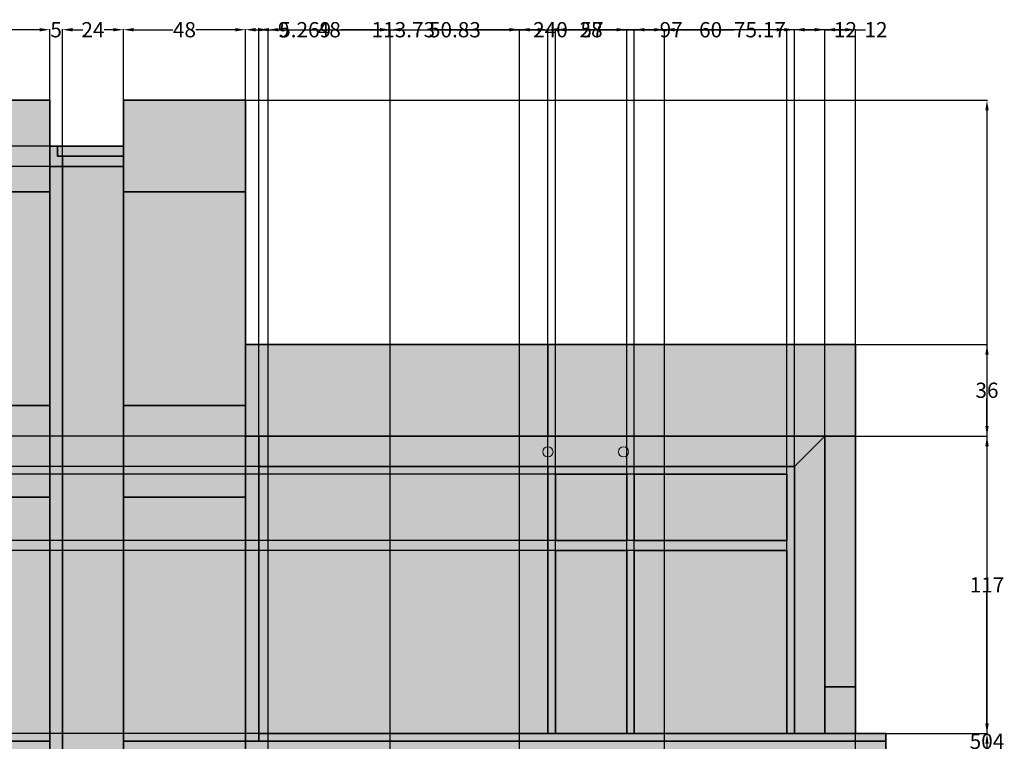
# Model space of a CAD drawing. Units: inches. Extents: x 221 to 874, y 171 to 738.
# Tile 11 of 11: x 452 to 840, y 455 to 738. Entities that reach past the tile are written whole.
import ezdxf

# ---------------------------------------------------------------- set-up
doc = ezdxf.new("R2010")
doc.units = ezdxf.units.IN
doc.header["$MEASUREMENT"] = 0
for name, color, linetype, lineweight in [('A-ANNO-DIMS', 2, 'Continuous', 18), ('A-ELEV', 7, 'Continuous', 35), ('A-ELEV-PATT', 8, 'Continuous', 13), ('E-LITE', 2, 'Continuous', 18)]:
    doc.layers.add(name, color=color, linetype=linetype, lineweight=lineweight)
doc.styles.get("Standard").update_dxf_attribs({"font": 'arial.ttf'})
doc.dimstyles.get("Standard").update_dxf_attribs({"dimtxt": 6, "dimasz": 4, "dimexe": 0.18, "dimexo": 0.0625, "dimgap": 0.09, "dimtad": 0, "dimtih": 1, "dimtoh": 1, "dimdec": 0, "dimzin": 0, "dimdsep": 46, "dimlunit": 3, "dimtxsty": 'Standard', "dimcen": 0.09, "dimadec": 0, "dimazin": 0, "dimtfac": 1, "dimtdec": 0, "dimtofl": 0, "dimtmove": 0, "dimatfit": 3, "dimfxl": 1, "dimtolj": 1, "dimtzin": 0, "dimarcsym": 0})

# ---------------------------------------------------------------- blocks, each defined once
blk = doc.blocks.new('*D21')
at = {"layer": 'A-ANNO-DIMS', "color": 0, "lineweight": -2, "transparency": 16777216}
for p, q in [((541.14, 706.72), (833.01, 706.72)), ((832.83, 702.72), (832.83, 457.87)), ((832.83, 206.72), (832.83, 451.56)), ((805.14, 202.72), (833.01, 202.72))]:
    blk.add_line(p, q, dxfattribs=at)
at = {"layer": 'A-ANNO-DIMS', "color": 0, "transparency": 16777216}
for points in [[(832.16, 702.72), (833.5, 702.72), (832.83, 706.72)], [(832.16, 206.72), (833.5, 206.72), (832.83, 202.72)]]:
    blk.add_solid(points, dxfattribs=at)
at = {"layer": 'Defpoints', "color": 0, "transparency": 16777216}
for p in [(541.08, 706.72), (832.83, 706.72), (805.08, 202.72)]:
    blk.add_point(p, dxfattribs=at)
at = {"layer": 'A-ANNO-DIMS', "color": 0, "transparency": 16777216, "insert": (832.83, 454.72), "char_height": 6, "attachment_point": 5}
blk.add_mtext('\\A1;504', dxfattribs=at)
blk = doc.blocks.new('*D24')
at = {"layer": 'A-ANNO-DIMS', "color": 0, "lineweight": -2, "transparency": 16777216}
for p, q in [((406.08, 706.78), (406.08, 734.65)), ((410.08, 734.47), (430.69, 734.47)), ((460.08, 734.47), (439.47, 734.47)), ((464.08, 706.78), (464.08, 734.65))]:
    blk.add_line(p, q, dxfattribs=at)
at = {"layer": 'A-ANNO-DIMS', "color": 0, "transparency": 16777216}
for points in [[(410.08, 735.13), (410.08, 733.8), (406.08, 734.47)], [(460.08, 735.13), (460.08, 733.8), (464.08, 734.47)]]:
    blk.add_solid(points, dxfattribs=at)
at = {"layer": 'Defpoints', "color": 0, "transparency": 16777216}
for p in [(464.08, 734.47), (406.08, 706.72), (464.08, 706.72)]:
    blk.add_point(p, dxfattribs=at)
at = {"layer": 'A-ANNO-DIMS', "color": 0, "transparency": 16777216, "insert": (435.08, 734.47), "char_height": 6, "attachment_point": 5}
blk.add_mtext('\\A1;58', dxfattribs=at)
blk = doc.blocks.new('*D25')
at = {"layer": 'A-ANNO-DIMS', "color": 0, "lineweight": -2, "transparency": 16777216}
for p, q in [((460.08, 734.47), (456.08, 734.47)), ((464.08, 680.78), (464.08, 734.65)), ((469.08, 680.78), (469.08, 734.65)), ((473.08, 734.47), (477.08, 734.47))]:
    blk.add_line(p, q, dxfattribs=at)
at = {"layer": 'A-ANNO-DIMS', "color": 0, "transparency": 16777216}
for points in [[(460.08, 735.13), (460.08, 733.8), (464.08, 734.47)], [(473.08, 735.13), (473.08, 733.8), (469.08, 734.47)]]:
    blk.add_solid(points, dxfattribs=at)
at = {"layer": 'Defpoints', "color": 0, "transparency": 16777216}
for p in [(469.08, 734.47), (464.08, 680.72), (469.08, 680.72)]:
    blk.add_point(p, dxfattribs=at)
at = {"layer": 'A-ANNO-DIMS', "color": 0, "transparency": 16777216, "insert": (466.58, 734.47), "char_height": 6, "attachment_point": 5}
blk.add_mtext('\\A1;5', dxfattribs=at)
blk = doc.blocks.new('*D26')
at = {"layer": 'A-ANNO-DIMS', "color": 0, "lineweight": -2, "transparency": 16777216}
for p, q in [((469.08, 680.78), (469.08, 734.65)), ((473.08, 734.47), (476.65, 734.47)), ((489.08, 734.47), (485.5, 734.47)), ((493.08, 680.78), (493.08, 734.65))]:
    blk.add_line(p, q, dxfattribs=at)
at = {"layer": 'A-ANNO-DIMS', "color": 0, "transparency": 16777216}
for points in [[(473.08, 735.13), (473.08, 733.8), (469.08, 734.47)], [(489.08, 735.13), (489.08, 733.8), (493.08, 734.47)]]:
    blk.add_solid(points, dxfattribs=at)
at = {"layer": 'Defpoints', "color": 0, "transparency": 16777216}
for p in [(493.08, 734.47), (469.08, 680.72), (493.08, 680.72)]:
    blk.add_point(p, dxfattribs=at)
at = {"layer": 'A-ANNO-DIMS', "color": 0, "transparency": 16777216, "insert": (481.08, 734.47), "char_height": 6, "attachment_point": 5}
blk.add_mtext('\\A1;24', dxfattribs=at)
blk = doc.blocks.new('*D27')
at = {"layer": 'A-ANNO-DIMS', "color": 0, "lineweight": -2, "transparency": 16777216}
for p, q in [((493.08, 706.78), (493.08, 734.65)), ((497.08, 734.47), (512.56, 734.47)), ((537.08, 734.47), (521.59, 734.47)), ((541.08, 706.78), (541.08, 734.65))]:
    blk.add_line(p, q, dxfattribs=at)
at = {"layer": 'A-ANNO-DIMS', "color": 0, "transparency": 16777216}
for points in [[(497.08, 735.13), (497.08, 733.8), (493.08, 734.47)], [(537.08, 735.13), (537.08, 733.8), (541.08, 734.47)]]:
    blk.add_solid(points, dxfattribs=at)
at = {"layer": 'Defpoints', "color": 0, "transparency": 16777216}
for p in [(541.08, 734.47), (493.08, 706.72), (541.08, 706.72)]:
    blk.add_point(p, dxfattribs=at)
at = {"layer": 'A-ANNO-DIMS', "color": 0, "transparency": 16777216, "insert": (517.08, 734.47), "char_height": 6, "attachment_point": 5}
blk.add_mtext('\\A1;48', dxfattribs=at)
blk = doc.blocks.new('*D28')
at = {"layer": 'A-ANNO-DIMS', "color": 0, "lineweight": -2, "transparency": 16777216}
for p, q in [((541.08, 706.78), (541.08, 734.65)), ((545.08, 734.47), (654.32, 734.47)), ((777.08, 734.47), (667.84, 734.47)), ((781.08, 610.78), (781.08, 734.65))]:
    blk.add_line(p, q, dxfattribs=at)
at = {"layer": 'A-ANNO-DIMS', "color": 0, "transparency": 16777216}
for points in [[(545.08, 735.13), (545.08, 733.8), (541.08, 734.47)], [(777.08, 735.13), (777.08, 733.8), (781.08, 734.47)]]:
    blk.add_solid(points, dxfattribs=at)
at = {"layer": 'Defpoints', "color": 0, "transparency": 16777216}
for p in [(781.08, 734.47), (541.08, 706.72), (781.08, 610.72)]:
    blk.add_point(p, dxfattribs=at)
at = {"layer": 'A-ANNO-DIMS', "color": 0, "transparency": 16777216, "insert": (661.08, 734.47), "char_height": 6, "attachment_point": 5}
blk.add_mtext('\\A1;240', dxfattribs=at)
blk = doc.blocks.new('*D40')
at = {"layer": 'A-ANNO-DIMS', "color": 0, "lineweight": -2, "transparency": 16777216}
for p, q in [((231.54, 692.72), (231.54, 696.72)), ((464.02, 688.72), (231.36, 688.72)), ((464.02, 680.72), (231.36, 680.72)), ((231.54, 676.72), (231.54, 672.72))]:
    blk.add_line(p, q, dxfattribs=at)
at = {"layer": 'A-ANNO-DIMS', "color": 0, "transparency": 16777216}
for points in [[(230.88, 692.72), (232.21, 692.72), (231.54, 688.72)], [(230.88, 676.72), (232.21, 676.72), (231.54, 680.72)]]:
    blk.add_solid(points, dxfattribs=at)
at = {"layer": 'Defpoints', "color": 0, "transparency": 16777216}
for p in [(231.54, 688.72), (464.08, 688.72), (464.08, 680.72)]:
    blk.add_point(p, dxfattribs=at)
at = {"layer": 'A-ANNO-DIMS', "color": 0, "transparency": 16777216, "insert": (231.54, 684.72), "char_height": 6, "attachment_point": 5}
blk.add_mtext('\\A1;8', dxfattribs=at)
blk = doc.blocks.new('*D41')
at = {"layer": 'A-ANNO-DIMS', "color": 0, "lineweight": -2, "transparency": 16777216}
for p, q in [((537.08, 734.47), (533.08, 734.47)), ((541.08, 574.78), (541.08, 734.65)), ((546.35, 574.78), (546.35, 734.65)), ((550.35, 734.47), (554.35, 734.47))]:
    blk.add_line(p, q, dxfattribs=at)
at = {"layer": 'A-ANNO-DIMS', "color": 0, "transparency": 16777216}
for points in [[(537.08, 735.13), (537.08, 733.8), (541.08, 734.47)], [(550.35, 735.13), (550.35, 733.8), (546.35, 734.47)]]:
    blk.add_solid(points, dxfattribs=at)
at = {"layer": 'Defpoints', "color": 0, "transparency": 16777216}
for p in [(546.35, 734.47), (541.08, 574.72), (546.35, 574.72)]:
    blk.add_point(p, dxfattribs=at)
at = {"layer": 'A-ANNO-DIMS', "color": 0, "transparency": 16777216, "insert": (564.57, 734.47), "char_height": 6, "attachment_point": 5}
blk.add_mtext('\\A1;5.269', dxfattribs=at)
blk = doc.blocks.new('*D42')
at = {"layer": 'A-ANNO-DIMS', "color": 0, "lineweight": -2, "transparency": 16777216}
for p, q in [((546.35, 574.78), (546.35, 734.65)), ((550.35, 734.47), (590.95, 734.47)), ((656.08, 734.47), (615.48, 734.47)), ((660.08, 562.78), (660.08, 734.65))]:
    blk.add_line(p, q, dxfattribs=at)
at = {"layer": 'A-ANNO-DIMS', "color": 0, "transparency": 16777216}
for points in [[(550.35, 735.13), (550.35, 733.8), (546.35, 734.47)], [(656.08, 735.13), (656.08, 733.8), (660.08, 734.47)]]:
    blk.add_solid(points, dxfattribs=at)
at = {"layer": 'Defpoints', "color": 0, "transparency": 16777216}
for p in [(660.08, 734.47), (546.35, 574.72), (660.08, 562.72)]:
    blk.add_point(p, dxfattribs=at)
at = {"layer": 'A-ANNO-DIMS', "color": 0, "transparency": 16777216, "insert": (603.21, 734.47), "char_height": 6, "attachment_point": 5}
blk.add_mtext('\\A1;113.73', dxfattribs=at)
blk = doc.blocks.new('*D43')
at = {"layer": 'A-ANNO-DIMS', "color": 0, "lineweight": -2, "transparency": 16777216}
for p, q in [((660.08, 562.78), (660.08, 734.65)), ((664.08, 734.47), (704.19, 734.47)), ((753.08, 734.47), (712.97, 734.47)), ((757.08, 562.78), (757.08, 734.65))]:
    blk.add_line(p, q, dxfattribs=at)
at = {"layer": 'A-ANNO-DIMS', "color": 0, "transparency": 16777216}
for points in [[(664.08, 735.13), (664.08, 733.8), (660.08, 734.47)], [(753.08, 735.13), (753.08, 733.8), (757.08, 734.47)]]:
    blk.add_solid(points, dxfattribs=at)
at = {"layer": 'Defpoints', "color": 0, "transparency": 16777216}
for p in [(757.08, 734.47), (660.08, 562.72), (757.08, 562.72)]:
    blk.add_point(p, dxfattribs=at)
at = {"layer": 'A-ANNO-DIMS', "color": 0, "transparency": 16777216, "insert": (708.58, 734.47), "char_height": 6, "attachment_point": 5}
blk.add_mtext('\\A1;97', dxfattribs=at)
blk = doc.blocks.new('*D44')
at = {"layer": 'A-ANNO-DIMS', "color": 0, "lineweight": -2, "transparency": 16777216}
for p, q in [((757.08, 562.78), (757.08, 734.65)), ((761.08, 734.47), (765.08, 734.47)), ((769.08, 574.78), (769.08, 734.65)), ((769.08, 734.47), (773.08, 734.47))]:
    blk.add_line(p, q, dxfattribs=at)
at = {"layer": 'A-ANNO-DIMS', "color": 0, "transparency": 16777216}
for points in [[(761.08, 735.13), (761.08, 733.8), (757.08, 734.47)], [(765.08, 735.13), (765.08, 733.8), (769.08, 734.47)]]:
    blk.add_solid(points, dxfattribs=at)
at = {"layer": 'Defpoints', "color": 0, "transparency": 16777216}
for p in [(769.08, 734.47), (769.08, 574.72), (757.08, 562.72)]:
    blk.add_point(p, dxfattribs=at)
at = {"layer": 'A-ANNO-DIMS', "color": 0, "transparency": 16777216, "insert": (777.15, 734.47), "char_height": 6, "attachment_point": 5}
blk.add_mtext('\\A1;12', dxfattribs=at)
blk = doc.blocks.new('*D45')
at = {"layer": 'A-ANNO-DIMS', "color": 0, "lineweight": -2, "transparency": 16777216}
for p, q in [((769.08, 574.78), (769.08, 734.65)), ((773.08, 734.47), (777.08, 734.47)), ((781.08, 574.78), (781.08, 734.65)), ((781.08, 734.47), (785.08, 734.47))]:
    blk.add_line(p, q, dxfattribs=at)
at = {"layer": 'A-ANNO-DIMS', "color": 0, "transparency": 16777216}
for points in [[(773.08, 735.13), (773.08, 733.8), (769.08, 734.47)], [(777.08, 735.13), (777.08, 733.8), (781.08, 734.47)]]:
    blk.add_solid(points, dxfattribs=at)
at = {"layer": 'Defpoints', "color": 0, "transparency": 16777216}
for p in [(781.08, 734.47), (769.08, 574.72), (781.08, 574.72)]:
    blk.add_point(p, dxfattribs=at)
at = {"layer": 'A-ANNO-DIMS', "color": 0, "transparency": 16777216, "insert": (789.15, 734.47), "char_height": 6, "attachment_point": 5}
blk.add_mtext('\\A1;12', dxfattribs=at)
blk = doc.blocks.new('*D48')
at = {"layer": 'A-ANNO-DIMS', "color": 0, "lineweight": -2, "transparency": 16777216}
for p, q in [((793.14, 457.72), (833.01, 457.72)), ((832.83, 453.72), (832.83, 447.32)), ((832.83, 434.72), (832.83, 441.11)), ((793.14, 430.72), (833.01, 430.72))]:
    blk.add_line(p, q, dxfattribs=at)
at = {"layer": 'A-ANNO-DIMS', "color": 0, "transparency": 16777216}
for points in [[(832.16, 453.72), (833.5, 453.72), (832.83, 457.72)], [(832.16, 434.72), (833.5, 434.72), (832.83, 430.72)]]:
    blk.add_solid(points, dxfattribs=at)
at = {"layer": 'Defpoints', "color": 0, "transparency": 16777216}
for p in [(793.08, 457.72), (832.83, 457.72), (793.08, 430.72)]:
    blk.add_point(p, dxfattribs=at)
at = {"layer": 'A-ANNO-DIMS', "color": 0, "transparency": 16777216, "insert": (832.83, 444.22), "char_height": 6, "attachment_point": 5}
blk.add_mtext('\\A1;27', dxfattribs=at)
blk = doc.blocks.new('*D49')
at = {"layer": 'A-ANNO-DIMS', "color": 0, "lineweight": -2, "transparency": 16777216}
for p, q in [((781.14, 574.72), (833.01, 574.72)), ((832.83, 570.72), (832.83, 519.32)), ((832.83, 461.72), (832.83, 513.11)), ((781.14, 457.72), (833.01, 457.72))]:
    blk.add_line(p, q, dxfattribs=at)
at = {"layer": 'A-ANNO-DIMS', "color": 0, "transparency": 16777216}
for points in [[(832.16, 570.72), (833.5, 570.72), (832.83, 574.72)], [(832.16, 461.72), (833.5, 461.72), (832.83, 457.72)]]:
    blk.add_solid(points, dxfattribs=at)
at = {"layer": 'Defpoints', "color": 0, "transparency": 16777216}
for p in [(781.08, 574.72), (832.83, 574.72), (781.08, 457.72)]:
    blk.add_point(p, dxfattribs=at)
at = {"layer": 'A-ANNO-DIMS', "color": 0, "transparency": 16777216, "insert": (832.83, 516.22), "char_height": 6, "attachment_point": 5}
blk.add_mtext('\\A1;117', dxfattribs=at)
blk = doc.blocks.new('*D50')
at = {"layer": 'A-ANNO-DIMS', "color": 0, "lineweight": -2, "transparency": 16777216}
for p, q in [((781.14, 610.72), (833.01, 610.72)), ((832.83, 606.72), (832.83, 595.87)), ((832.83, 578.72), (832.83, 589.56)), ((781.14, 574.72), (833.01, 574.72))]:
    blk.add_line(p, q, dxfattribs=at)
at = {"layer": 'A-ANNO-DIMS', "color": 0, "transparency": 16777216}
for points in [[(832.16, 606.72), (833.5, 606.72), (832.83, 610.72)], [(832.16, 578.72), (833.5, 578.72), (832.83, 574.72)]]:
    blk.add_solid(points, dxfattribs=at)
at = {"layer": 'Defpoints', "color": 0, "transparency": 16777216}
for p in [(781.08, 610.72), (832.83, 610.72), (781.08, 574.72)]:
    blk.add_point(p, dxfattribs=at)
at = {"layer": 'A-ANNO-DIMS', "color": 0, "transparency": 16777216, "insert": (832.83, 592.72), "char_height": 6, "attachment_point": 5}
blk.add_mtext('\\A1;36', dxfattribs=at)
blk = doc.blocks.new('*D51')
at = {"layer": 'A-ANNO-DIMS', "color": 0, "lineweight": -2, "transparency": 16777216}
for p, q in [((546.29, 562.72), (231.36, 562.72)), ((231.54, 558.72), (231.54, 513.37)), ((231.54, 461.72), (231.54, 507.06)), ((546.29, 457.72), (231.36, 457.72))]:
    blk.add_line(p, q, dxfattribs=at)
at = {"layer": 'A-ANNO-DIMS', "color": 0, "transparency": 16777216}
for points in [[(230.88, 558.72), (232.21, 558.72), (231.54, 562.72)], [(230.88, 461.72), (232.21, 461.72), (231.54, 457.72)]]:
    blk.add_solid(points, dxfattribs=at)
at = {"layer": 'Defpoints', "color": 0, "transparency": 16777216}
for p in [(231.54, 562.72), (546.35, 562.72), (546.35, 457.72)]:
    blk.add_point(p, dxfattribs=at)
at = {"layer": 'A-ANNO-DIMS', "color": 0, "transparency": 16777216, "insert": (231.54, 510.22), "char_height": 6, "attachment_point": 5}
blk.add_mtext('\\A1;105', dxfattribs=at)
blk = doc.blocks.new('*D52')
at = {"layer": 'A-ANNO-DIMS', "color": 0, "lineweight": -2, "transparency": 16777216}
for p, q in [((231.54, 574.72), (231.54, 578.72)), ((231.54, 578.72), (235.54, 578.72)), ((546.29, 574.72), (231.36, 574.72)), ((231.54, 566.72), (231.54, 570.72)), ((546.29, 562.72), (231.36, 562.72))]:
    blk.add_line(p, q, dxfattribs=at)
at = {"layer": 'A-ANNO-DIMS', "color": 0, "transparency": 16777216}
for points in [[(230.88, 570.72), (232.21, 570.72), (231.54, 574.72)], [(230.88, 566.72), (232.21, 566.72), (231.54, 562.72)]]:
    blk.add_solid(points, dxfattribs=at)
at = {"layer": 'Defpoints', "color": 0, "transparency": 16777216}
for p in [(231.54, 574.72), (546.35, 574.72), (546.35, 562.72)]:
    blk.add_point(p, dxfattribs=at)
at = {"layer": 'A-ANNO-DIMS', "color": 0, "transparency": 16777216, "insert": (239.62, 578.72), "char_height": 6, "attachment_point": 5}
blk.add_mtext('\\A1;12', dxfattribs=at)
blk = doc.blocks.new('*D53')
at = {"layer": 'A-ANNO-DIMS', "color": 0, "lineweight": -2, "transparency": 16777216}
for p, q in [((663.08, 529.78), (663.08, 734.65)), ((667.08, 734.47), (672.63, 734.47)), ((687.08, 734.47), (681.52, 734.47)), ((691.08, 529.78), (691.08, 734.65))]:
    blk.add_line(p, q, dxfattribs=at)
at = {"layer": 'A-ANNO-DIMS', "color": 0, "transparency": 16777216}
for points in [[(667.08, 735.13), (667.08, 733.8), (663.08, 734.47)], [(687.08, 735.13), (687.08, 733.8), (691.08, 734.47)]]:
    blk.add_solid(points, dxfattribs=at)
at = {"layer": 'Defpoints', "color": 0, "transparency": 16777216}
for p in [(691.08, 734.47), (663.08, 529.72), (691.08, 529.72)]:
    blk.add_point(p, dxfattribs=at)
at = {"layer": 'A-ANNO-DIMS', "color": 0, "transparency": 16777216, "insert": (677.08, 734.47), "char_height": 6, "attachment_point": 5}
blk.add_mtext('\\A1;28', dxfattribs=at)
blk = doc.blocks.new('*D54')
at = {"layer": 'A-ANNO-DIMS', "color": 0, "lineweight": -2, "transparency": 16777216}
for p, q in [((694.08, 529.78), (694.08, 734.65)), ((698.08, 734.47), (719.69, 734.47)), ((750.08, 734.47), (728.47, 734.47)), ((754.08, 529.78), (754.08, 734.65))]:
    blk.add_line(p, q, dxfattribs=at)
at = {"layer": 'A-ANNO-DIMS', "color": 0, "transparency": 16777216}
for points in [[(698.08, 735.13), (698.08, 733.8), (694.08, 734.47)], [(750.08, 735.13), (750.08, 733.8), (754.08, 734.47)]]:
    blk.add_solid(points, dxfattribs=at)
at = {"layer": 'Defpoints', "color": 0, "transparency": 16777216}
for p in [(754.08, 734.47), (694.08, 529.72), (754.08, 529.72)]:
    blk.add_point(p, dxfattribs=at)
at = {"layer": 'A-ANNO-DIMS', "color": 0, "transparency": 16777216, "insert": (724.08, 734.47), "char_height": 6, "attachment_point": 5}
blk.add_mtext('\\A1;60', dxfattribs=at)
blk = doc.blocks.new('*D55')
at = {"layer": 'A-ANNO-DIMS', "color": 0, "lineweight": -2, "transparency": 16777216}
for p, q in [((754.02, 559.72), (231.36, 559.72)), ((231.54, 555.72), (231.54, 549.87)), ((231.54, 537.72), (231.54, 543.56)), ((754.02, 533.72), (231.36, 533.72))]:
    blk.add_line(p, q, dxfattribs=at)
at = {"layer": 'A-ANNO-DIMS', "color": 0, "transparency": 16777216}
for points in [[(230.88, 555.72), (232.21, 555.72), (231.54, 559.72)], [(230.88, 537.72), (232.21, 537.72), (231.54, 533.72)]]:
    blk.add_solid(points, dxfattribs=at)
at = {"layer": 'Defpoints', "color": 0, "transparency": 16777216}
for p in [(231.54, 559.72), (754.08, 559.72), (754.08, 533.72)]:
    blk.add_point(p, dxfattribs=at)
at = {"layer": 'A-ANNO-DIMS', "color": 0, "transparency": 16777216, "insert": (231.54, 546.72), "char_height": 6, "attachment_point": 5}
blk.add_mtext('\\A1;26', dxfattribs=at)
blk = doc.blocks.new('*D56')
at = {"layer": 'A-ANNO-DIMS', "color": 0, "lineweight": -2, "transparency": 16777216}
for p, q in [((754.02, 529.72), (231.36, 529.72)), ((231.54, 525.72), (231.54, 496.82)), ((231.54, 461.72), (231.54, 490.61)), ((754.02, 457.72), (231.36, 457.72))]:
    blk.add_line(p, q, dxfattribs=at)
at = {"layer": 'A-ANNO-DIMS', "color": 0, "transparency": 16777216}
for points in [[(230.88, 525.72), (232.21, 525.72), (231.54, 529.72)], [(230.88, 461.72), (232.21, 461.72), (231.54, 457.72)]]:
    blk.add_solid(points, dxfattribs=at)
at = {"layer": 'Defpoints', "color": 0, "transparency": 16777216}
for p in [(231.54, 529.72), (754.08, 529.72), (754.08, 457.72)]:
    blk.add_point(p, dxfattribs=at)
at = {"layer": 'A-ANNO-DIMS', "color": 0, "transparency": 16777216, "insert": (231.54, 493.72), "char_height": 6, "attachment_point": 5}
blk.add_mtext('\\A1;72', dxfattribs=at)
blk = doc.blocks.new('*D57')
at = {"layer": 'A-ANNO-DIMS', "color": 0, "lineweight": -2, "transparency": 16777216}
for p, q in [((541.08, 377.16), (541.08, 734.65)), ((545.08, 734.47), (546.08, 734.47)), ((550.08, 377.16), (550.08, 734.65)), ((550.08, 734.47), (554.08, 734.47))]:
    blk.add_line(p, q, dxfattribs=at)
at = {"layer": 'A-ANNO-DIMS', "color": 0, "transparency": 16777216}
for points in [[(545.08, 735.13), (545.08, 733.8), (541.08, 734.47)], [(546.08, 735.13), (546.08, 733.8), (550.08, 734.47)]]:
    blk.add_solid(points, dxfattribs=at)
at = {"layer": 'Defpoints', "color": 0, "transparency": 16777216}
for p in [(550.08, 734.47), (541.08, 377.1), (550.08, 377.1)]:
    blk.add_point(p, dxfattribs=at)
at = {"layer": 'A-ANNO-DIMS', "color": 0, "transparency": 16777216, "insert": (556.14, 734.47), "char_height": 6, "attachment_point": 5}
blk.add_mtext('\\A1;9', dxfattribs=at)
blk = doc.blocks.new('*D58')
at = {"layer": 'A-ANNO-DIMS', "color": 0, "lineweight": -2, "transparency": 16777216}
for p, q in [((550.08, 377.16), (550.08, 734.65)), ((554.08, 734.47), (569.56, 734.47)), ((594.08, 734.47), (578.59, 734.47)), ((598.08, 377.16), (598.08, 734.65))]:
    blk.add_line(p, q, dxfattribs=at)
at = {"layer": 'A-ANNO-DIMS', "color": 0, "transparency": 16777216}
for points in [[(554.08, 735.13), (554.08, 733.8), (550.08, 734.47)], [(594.08, 735.13), (594.08, 733.8), (598.08, 734.47)]]:
    blk.add_solid(points, dxfattribs=at)
at = {"layer": 'Defpoints', "color": 0, "transparency": 16777216}
for p in [(598.08, 734.47), (550.08, 377.1), (598.08, 377.1)]:
    blk.add_point(p, dxfattribs=at)
at = {"layer": 'A-ANNO-DIMS', "color": 0, "transparency": 16777216, "insert": (574.08, 734.47), "char_height": 6, "attachment_point": 5}
blk.add_mtext('\\A1;48', dxfattribs=at)
blk = doc.blocks.new('*D59')
at = {"layer": 'A-ANNO-DIMS', "color": 0, "lineweight": -2, "transparency": 16777216}
for p, q in [((598.08, 377.16), (598.08, 734.65)), ((602.08, 734.47), (613.28, 734.47)), ((644.91, 734.47), (633.71, 734.47)), ((648.91, 377.16), (648.91, 734.65))]:
    blk.add_line(p, q, dxfattribs=at)
at = {"layer": 'A-ANNO-DIMS', "color": 0, "transparency": 16777216}
for points in [[(602.08, 735.13), (602.08, 733.8), (598.08, 734.47)], [(644.91, 735.13), (644.91, 733.8), (648.91, 734.47)]]:
    blk.add_solid(points, dxfattribs=at)
at = {"layer": 'Defpoints', "color": 0, "transparency": 16777216}
for p in [(648.91, 734.47), (598.08, 377.1), (648.91, 377.1)]:
    blk.add_point(p, dxfattribs=at)
at = {"layer": 'A-ANNO-DIMS', "color": 0, "transparency": 16777216, "insert": (623.49, 734.47), "char_height": 6, "attachment_point": 5}
blk.add_mtext('\\A1;50.83', dxfattribs=at)
blk = doc.blocks.new('*D60')
at = {"layer": 'A-ANNO-DIMS', "color": 0, "lineweight": -2, "transparency": 16777216}
for p, q in [((648.91, 377.16), (648.91, 734.65)), ((652.91, 734.47), (673.02, 734.47)), ((701.91, 734.47), (681.8, 734.47)), ((705.91, 377.16), (705.91, 734.65))]:
    blk.add_line(p, q, dxfattribs=at)
at = {"layer": 'A-ANNO-DIMS', "color": 0, "transparency": 16777216}
for points in [[(652.91, 735.13), (652.91, 733.8), (648.91, 734.47)], [(701.91, 735.13), (701.91, 733.8), (705.91, 734.47)]]:
    blk.add_solid(points, dxfattribs=at)
at = {"layer": 'Defpoints', "color": 0, "transparency": 16777216}
for p in [(705.91, 734.47), (648.91, 377.1), (705.91, 377.1)]:
    blk.add_point(p, dxfattribs=at)
at = {"layer": 'A-ANNO-DIMS', "color": 0, "transparency": 16777216, "insert": (677.41, 734.47), "char_height": 6, "attachment_point": 5}
blk.add_mtext('\\A1;57', dxfattribs=at)
blk = doc.blocks.new('*D61')
at = {"layer": 'A-ANNO-DIMS', "color": 0, "lineweight": -2, "transparency": 16777216}
for p, q in [((705.91, 377.16), (705.91, 734.65)), ((709.91, 734.47), (733.31, 734.47)), ((777.08, 734.47), (753.68, 734.47)), ((781.08, 377.16), (781.08, 734.65))]:
    blk.add_line(p, q, dxfattribs=at)
at = {"layer": 'A-ANNO-DIMS', "color": 0, "transparency": 16777216}
for points in [[(709.91, 735.13), (709.91, 733.8), (705.91, 734.47)], [(777.08, 735.13), (777.08, 733.8), (781.08, 734.47)]]:
    blk.add_solid(points, dxfattribs=at)
at = {"layer": 'Defpoints', "color": 0, "transparency": 16777216}
for p in [(781.08, 734.47), (705.91, 377.1), (781.08, 377.1)]:
    blk.add_point(p, dxfattribs=at)
at = {"layer": 'A-ANNO-DIMS', "color": 0, "transparency": 16777216, "insert": (743.49, 734.47), "char_height": 6, "attachment_point": 5}
blk.add_mtext('\\A1;75.17', dxfattribs=at)

msp = doc.modelspace()

# ---------------------------------------------------------------- hatches: boundary and pattern name
at = {"layer": 'A-ELEV-PATT'}
h = msp.add_hatch(color=256, dxfattribs=at)
h.dxf.hatch_style = 1
h.paths.add_polyline_path([(349.0786, 286.1996), (313.0786, 286.1996), (313.0786, 232.7164), (349.0786, 232.7164)])
h.paths.add_polyline_path([(464.0786, 286.1996), (406.0786, 286.1996), (406.0786, 232.7164), (464.0786, 232.7164)])
h.paths.add_polyline_path([(541.0786, 286.1996), (493.0786, 286.1996), (493.0786, 232.7164), (541.0786, 232.7164)])
h.paths.add_polyline_path([(541.0786, 370.7164), (493.0786, 370.7164), (493.0786, 286.1996), (541.0786, 286.1996)])
h.paths.add_polyline_path([(464.0786, 370.7164), (406.0786, 370.7164), (406.0786, 286.1996), (464.0786, 286.1996)])
h.paths.add_polyline_path([(349.0786, 370.7164), (313.0786, 370.7164), (313.0786, 286.1996), (349.0786, 286.1996)])
h.paths.add_polyline_path([(349.0786, 454.7164), (313.0786, 454.7164), (313.0786, 370.7164), (349.0786, 370.7164)])
h.paths.add_polyline_path([(464.0786, 454.7164), (406.0786, 454.7164), (406.0786, 370.7164), (464.0786, 370.7164)])
h.paths.add_polyline_path([(541.0786, 418.7164), (541.0786, 454.7164), (493.0786, 454.7164), (493.0786, 370.7164), (541.0786, 370.7164)])
h.paths.add_polyline_path([(541.0786, 550.7164), (493.0786, 550.7164), (493.0786, 454.7164), (541.0786, 454.7164)])
h.paths.add_polyline_path([(464.0786, 550.7164), (406.0786, 550.7164), (406.0786, 454.7164), (464.0786, 454.7164)])
h.paths.add_polyline_path([(349.0786, 550.7164), (313.0786, 550.7164), (313.0786, 454.7164), (349.0786, 454.7164)])
h.paths.add_polyline_path([(349.0786, 586.7164), (313.0786, 586.7164), (313.0786, 550.7164), (349.0786, 550.7164)])
h.paths.add_polyline_path([(464.0786, 586.7164), (406.0786, 586.7164), (406.0786, 550.7164), (464.0786, 550.7164)])
h.paths.add_polyline_path([(541.0786, 574.7164), (541.0786, 586.7164), (493.0786, 586.7164), (493.0786, 550.7164), (541.0786, 550.7164)])
h.paths.add_polyline_path([(541.0786, 670.7164), (493.0786, 670.7164), (493.0786, 586.7164), (541.0786, 586.7164)])
h.paths.add_polyline_path([(464.0786, 670.7164), (406.0786, 670.7164), (406.0786, 586.7164), (464.0786, 586.7164)])
h.paths.add_polyline_path([(349.0786, 670.7164), (313.0786, 670.7164), (313.0786, 586.7164), (349.0786, 586.7164)])
h.paths.add_polyline_path([(406.0786, 706.7164), (313.0786, 706.7164), (313.0786, 670.7164), (349.0786, 670.7164), (406.0786, 670.7164)])
h.paths.add_polyline_path([(464.0786, 706.7164), (406.0786, 706.7164), (406.0786, 670.7164), (464.0786, 670.7164)])
h.paths.add_polyline_path([(541.0786, 706.7164), (493.0786, 706.7164), (493.0786, 688.7164), (493.0786, 670.7164), (541.0786, 670.7164)])
h.paths.add_polyline_path([(660.0786, 610.7164), (541.0786, 610.7164), (541.0786, 586.7164), (541.0786, 574.7164), (660.0786, 574.7164)])
h.paths.add_polyline_path([(781.0786, 610.7164), (660.0786, 610.7164), (660.0786, 574.7164), (769.0786, 574.7164), (781.0786, 574.7164)])
h.paths.add_polyline_path([(781.0786, 574.7164), (769.0786, 574.7164), (769.0786, 476.1199), (781.0786, 476.1199)])
h.paths.add_polyline_path([(781.0786, 476.1199), (769.0786, 476.1199), (769.0786, 457.7164), (781.0786, 457.7164)])
h.paths.add_polyline_path([(781.0786, 377.1023), (705.9097, 377.1023), (705.9097, 286.1996), (781.0786, 286.1996)])
h.paths.add_polyline_path([(741.9618, 338.8486), (756.9618, 338.8486), (756.9618, 329.8486), (741.9618, 329.8486)], flags=16)
h.paths.add_polyline_path([(648.9097, 377.1023), (598.0786, 377.1023), (598.0786, 286.1996), (648.9097, 286.1996)])
h.paths.add_polyline_path([(781.0786, 286.1996), (705.9097, 286.1996), (705.9097, 280.7164), (648.9097, 280.7164), (648.9097, 286.1996), (598.0786, 286.1996), (598.0786, 280.7164), (550.0786, 280.7164), (550.0786, 286.1996), (541.0786, 286.1996), (541.0786, 274.7164), (781.0786, 274.7164)])
h.paths.add_polyline_path([(660.0786, 562.7164), (546.3477, 562.7164), (546.3477, 457.7164), (660.0786, 457.7164)])
h = msp.add_hatch(color=256, dxfattribs=at)
h.set_gradient(color1=(254, 204, 102), name='CYLINDER')
h.paths.add_polyline_path([(464.0786, 680.7164), (469.0786, 680.7164), (469.0786, 684.7164), (467.0786, 684.7164), (467.0786, 688.7164), (464.0786, 688.7164)])
h = msp.add_hatch(color=256, dxfattribs=at)
h.paths.add_polyline_path([(493.0786, 688.7164), (467.0786, 688.7164), (467.0786, 684.7164), (469.0786, 684.7164), (493.0786, 684.7164)])
h.paths.add_polyline_path([(493.0786, 684.7164), (469.0786, 684.7164), (469.0786, 680.7164), (493.0786, 680.7164)])
h = msp.add_hatch(color=256, dxfattribs=at)
h.set_gradient(color1=(255, 236, 199), name='CYLINDER')
h.paths.add_polyline_path([(469.0786, 680.7164), (464.0786, 680.7164), (464.0786, 232.7164), (469.0786, 232.7164)])
h = msp.add_hatch(color=256, dxfattribs=at)
h.set_gradient(color1=(147, 149, 152), color2=(254, 234, 185), name='CYLINDER')
h.paths.add_polyline_path([(469.0786, 430.7164), (493.0786, 430.7164), (493.0786, 680.7164), (469.0786, 680.7164)])
h = msp.add_hatch(color=256, dxfattribs=at)
h.set_gradient(color1=(254, 234, 185), name='CYLINDER')
h.paths.add_polyline_path([(541.0786, 454.7164), (546.3477, 454.7164), (546.3477, 574.7164), (541.0786, 574.7164)])
h = msp.add_hatch(color=256, dxfattribs=at)
h.set_gradient(color1=(209, 204, 163), color2=(80, 81, 83), rotation=90, name='INVCYLINDER')
h.paths.add_polyline_path([(546.3477, 574.7164), (546.3477, 562.7164), (660.0786, 562.7164), (757.0786, 562.7164), (769.0786, 574.7164)])
h.paths.add_polyline_path([(662.0861, 568.5315, -1), (658.0861, 568.5315, -1)], flags=16)
h.paths.add_polyline_path([(691.8096, 568.5315, -1), (687.8096, 568.5315, -1)], flags=16)
h = msp.add_hatch(color=256, dxfattribs=at)
h.set_gradient(color1=(209, 204, 163), color2=(147, 149, 152), name='INVCYLINDER')
h.paths.add_polyline_path([(757.0786, 457.7164), (769.0786, 457.7164), (769.0786, 574.7164), (757.0786, 562.7164)])
h = msp.add_hatch(color=256, dxfattribs=at)
h.paths.add_polyline_path([(662.0861, 568.5315, 1), (658.0861, 568.5315, 1)])
h.paths.add_polyline_path([(691.8096, 568.5315, 1), (687.8096, 568.5315, 1)])
h = msp.add_hatch(color=256, dxfattribs=at)
h.paths.add_polyline_path([(757.0786, 562.7164), (660.0786, 562.7164), (660.0786, 457.7164), (663.0786, 457.7164), (663.0786, 529.7164), (691.0786, 529.7164), (691.0786, 457.7164), (694.0786, 457.7164), (694.0786, 529.7164), (754.0786, 529.7164), (754.0786, 457.7164), (757.0786, 457.7164)])
h.paths.add_polyline_path([(754.0786, 533.7164), (694.0786, 533.7164), (694.0786, 559.7164), (754.0786, 559.7164)], flags=16)
h.paths.add_polyline_path([(691.0786, 533.7164), (663.0786, 533.7164), (663.0786, 559.7164), (691.0786, 559.7164)], flags=16)
h = msp.add_hatch(color=256, dxfattribs=at)
h.set_gradient(color1=(254, 234, 185), color2=(237, 203, 135), name='INVSPHERICAL')
h.paths.add_polyline_path([(691.0786, 533.7164), (691.0786, 559.7164), (663.0786, 559.7164), (663.0786, 533.7164)])
h = msp.add_hatch(color=256, dxfattribs=at)
h.set_gradient(color1=(254, 234, 185), color2=(147, 149, 152), name='INVCYLINDER')
h.paths.add_polyline_path([(754.0786, 529.7164), (694.0786, 529.7164), (694.0786, 457.7164), (754.0786, 457.7164)])
h.paths.add_polyline_path([(694.0786, 559.7164), (694.0786, 533.7164), (754.0786, 533.7164), (754.0786, 559.7164)])
h = msp.add_hatch(color=256, dxfattribs=at)
h.set_gradient(color1=(254, 234, 185), color2=(237, 203, 135), name='INVSPHERICAL')
h.paths.add_polyline_path([(663.0786, 457.7164), (691.0786, 457.7164), (691.0786, 529.7164), (663.0786, 529.7164)])
msp.add_hatch(color=256, dxfattribs=at).paths.add_polyline_path([(793.0786, 457.7164), (546.3477, 457.7164), (546.3477, 454.7164), (793.0786, 454.7164)])
h = msp.add_hatch(color=256, dxfattribs=at)
h.dxf.hatch_style = 1
h.paths.add_polyline_path([(793.0786, 441.595), (793.0786, 454.7164), (541.0786, 454.7164), (541.0786, 441.595)])

# ---------------------------------------------------------------- linework, layer by layer
at = {"layer": 'A-ELEV'}
for p, q in [((313.0786, 706.7164), (464.0786, 706.7164)), ((464.0786, 706.7164), (464.0786, 232.7164)), ((493.0786, 688.7164), (493.0786, 706.7164)), ((493.0786, 706.7164), (541.0786, 706.7164)), ((541.0786, 706.7164), (541.0786, 574.7164)), ((464.0786, 688.7164), (493.0786, 688.7164)), ((467.0786, 684.7164), (467.0786, 688.7164)), ((493.0786, 688.7164), (493.0786, 232.7164)), ((469.0786, 684.7164), (467.0786, 684.7164)), ((469.0786, 684.7164), (469.0786, 232.7164)), ((469.0786, 684.7164), (493.0786, 684.7164)), ((493.0786, 684.7164), (493.0786, 680.7164)), ((469.0786, 680.7164), (464.0786, 680.7164)), ((493.0786, 680.7164), (469.0786, 680.7164)), ((313.0786, 670.7164), (464.0786, 670.7164)), ((493.0786, 670.7164), (541.0786, 670.7164)), ((541.0786, 610.7164), (781.0786, 610.7164)), ((660.0786, 574.7164), (660.0786, 610.7164)), ((781.0786, 610.7164), (781.0786, 457.7164)), ((406.0786, 586.7164), (464.0786, 586.7164)), ((493.0786, 586.7164), (541.0786, 586.7164)), ((541.0786, 574.7164), (769.0786, 574.7164)), ((541.0786, 418.7164), (541.0786, 574.7164)), ((546.3477, 574.7164), (546.3477, 454.7164)), ((769.0786, 574.7164), (757.0786, 562.7164)), ((769.0786, 574.7164), (769.0786, 457.7164)), ((769.0786, 574.7164), (781.0786, 574.7164)), ((546.3477, 562.7164), (660.0786, 562.7164)), ((660.0786, 562.7164), (757.0786, 562.7164)), ((660.0786, 562.7164), (660.0786, 457.7164)), ((757.0786, 562.7164), (757.0786, 457.7164)), ((663.0786, 559.7164), (691.0786, 559.7164)), ((663.0786, 559.7164), (663.0786, 533.7164)), ((691.0786, 559.7164), (691.0786, 533.7164)), ((694.0786, 559.7164), (694.0786, 533.7164)), ((694.0786, 559.7164), (754.0786, 559.7164)), ((754.0786, 559.7164), (754.0786, 533.7164)), ((406.0786, 550.7164), (464.0786, 550.7164)), ((493.0786, 550.7164), (541.0786, 550.7164)), ((663.0786, 533.7164), (691.0786, 533.7164)), ((694.0786, 533.7164), (754.0786, 533.7164)), ((663.0786, 529.7164), (691.0786, 529.7164)), ((663.0786, 529.7164), (663.0786, 457.7164)), ((691.0786, 529.7164), (691.0786, 457.7164)), ((694.0786, 529.7164), (694.0786, 457.7164)), ((694.0786, 529.7164), (754.0786, 529.7164)), ((754.0786, 529.7164), (754.0786, 457.7164)), ((769.0786, 476.1199), (781.0786, 476.1199)), ((546.3477, 457.7164), (793.0786, 457.7164)), ((793.0786, 457.7164), (793.0786, 430.7164)), ((313.0786, 454.7164), (464.0786, 454.7164)), ((493.0786, 454.7164), (541.0786, 454.7164)), ((541.0786, 454.7164), (793.0786, 454.7164))]:
    msp.add_line(p, q, dxfattribs=at)
for points in [[(464.0786, 680.7164), (469.0786, 680.7164), (469.0786, 232.7164), (464.0786, 232.7164)], [(546.3477, 457.7164), (793.0786, 457.7164), (793.0786, 454.7164), (546.3477, 454.7164)]]:
    msp.add_lwpolyline(points, close=True, dxfattribs=at)
at = {"layer": 'E-LITE'}
for centre in [(660.0861, 568.5315), (689.8096, 568.5315)]:
    msp.add_circle(centre, 2, dxfattribs=at)

# ---------------------------------------------------------------- dimensions: what is measured, and where the dimension line sits
at = {"layer": 'A-ANNO-DIMS'}
for base, p1, p2, override, picture, middle in [((464.0786, 734.4664), (406.0786, 706.7164), (464.0786, 706.7164), {"dimdec": 0, "dimlfac": 1, "dimrnd": 0, "dimzin": 0, "dimdsep": 46, "dimlunit": 2}, '*D24', (435.0786, 734.4664)), ((469.0786, 734.4664), (464.0786, 680.7164), (469.0786, 680.7164), {"dimdec": 0, "dimlfac": 1, "dimrnd": 0, "dimzin": 0, "dimdsep": 46, "dimlunit": 2}, '*D25', (466.5786, 734.4664)), ((493.0786, 734.4664), (469.0786, 680.7164), (493.0786, 680.7164), {"dimdec": 0, "dimlfac": 1, "dimrnd": 0, "dimzin": 0, "dimdsep": 46, "dimlunit": 2}, '*D26', (481.0786, 734.4664)), ((541.0786, 734.4664), (493.0786, 706.7164), (541.0786, 706.7164), {"dimdec": 0, "dimlfac": 1, "dimrnd": 0, "dimzin": 0, "dimdsep": 46, "dimlunit": 2}, '*D27', (517.0786, 734.4664)), ((546.3477, 734.4664), (541.0786, 574.7164), (546.3477, 574.7164), {"dimdec": 3, "dimlfac": 1, "dimrnd": 0, "dimzin": 0, "dimdsep": 46, "dimlunit": 2}, '*D41', (564.5673, 734.4664)), ((781.0786, 734.4664), (541.0786, 706.7164), (781.0786, 610.7164), {"dimdec": 0, "dimlfac": 1, "dimrnd": 0, "dimzin": 0, "dimdsep": 46, "dimlunit": 2}, '*D28', (661.0786, 734.4664)), ((550.0786, 734.4664), (541.0786, 377.1023), (550.0786, 377.1023), {"dimdec": 0, "dimlfac": 1, "dimrnd": 0, "dimzin": 0, "dimdsep": 46, "dimlunit": 2}, '*D57', (556.1413, 734.4664)), ((660.0786, 734.4664), (546.3477, 574.7164), (660.0786, 562.7164), {"dimdec": 2, "dimlfac": 1, "dimrnd": 0, "dimzin": 0, "dimdsep": 46, "dimlunit": 2}, '*D42', (603.2132, 734.4664)), ((598.0786, 734.4664), (550.0786, 377.1023), (598.0786, 377.1023), {"dimdec": 0, "dimlfac": 1, "dimrnd": 0, "dimzin": 0, "dimdsep": 46, "dimlunit": 2}, '*D58', (574.0786, 734.4664)), ((648.9097, 734.4664), (598.0786, 377.1023), (648.9097, 377.1023), {"dimdec": 2, "dimlfac": 1, "dimrnd": 0, "dimzin": 0, "dimdsep": 46, "dimlunit": 2}, '*D59', (623.4941, 734.4664)), ((705.9097, 734.4664), (648.9097, 377.1023), (705.9097, 377.1023), {"dimdec": 0, "dimlfac": 1, "dimrnd": 0, "dimzin": 0, "dimdsep": 46, "dimlunit": 2}, '*D60', (677.4097, 734.4664)), ((757.0786, 734.4664), (660.0786, 562.7164), (757.0786, 562.7164), {"dimdec": 0, "dimlfac": 1, "dimrnd": 0, "dimzin": 0, "dimdsep": 46, "dimlunit": 2}, '*D43', (708.5786, 734.4664)), ((691.0786, 734.4664), (663.0786, 529.7164), (691.0786, 529.7164), {"dimdec": 0, "dimlfac": 1, "dimrnd": 0, "dimzin": 0, "dimdsep": 46, "dimlunit": 2}, '*D53', (677.0786, 734.4664)), ((754.0786, 734.4664), (694.0786, 529.7164), (754.0786, 529.7164), {"dimdec": 0, "dimlfac": 1, "dimrnd": 0, "dimzin": 0, "dimdsep": 46, "dimlunit": 2}, '*D54', (724.0786, 734.4664)), ((781.0786, 734.4664), (705.9097, 377.1023), (781.0786, 377.1023), {"dimdec": 2, "dimlfac": 1, "dimrnd": 0, "dimzin": 0, "dimdsep": 46, "dimlunit": 2}, '*D61', (743.4941, 734.4664)), ((769.0786, 734.4664), (757.0786, 562.7164), (769.0786, 574.7164), {"dimdec": 0, "dimlfac": 1, "dimrnd": 0, "dimzin": 0, "dimdsep": 46, "dimlunit": 2}, '*D44', (777.1529, 734.4664)), ((781.0786, 734.4664), (769.0786, 574.7164), (781.0786, 574.7164), {"dimdec": 0, "dimlfac": 1, "dimrnd": 0, "dimzin": 0, "dimdsep": 46, "dimlunit": 2}, '*D45', (789.1529, 734.4664))]:
    dim = msp.add_linear_dim(base=base, p1=p1, p2=p2, dimstyle='Standard', override=override, dxfattribs=at)
    dim.commit()
    dim.dimension.update_dxf_attribs({"geometry": picture, "text_midpoint": middle})
for base, p1, p2, picture, middle in [((832.8286, 706.7164), (805.0786, 202.7164), (541.0786, 706.7164), '*D21', (832.8286, 454.7164)), ((231.5426, 688.7164), (464.0786, 680.7164), (464.0786, 688.7164), '*D40', (231.5426, 684.7164)), ((832.8286, 610.7164), (781.0786, 574.7164), (781.0786, 610.7164), '*D50', (832.8286, 592.7164)), ((231.5426, 574.7164), (546.3477, 562.7164), (546.3477, 574.7164), '*D52', (239.6169, 578.7164)), ((832.8286, 574.7164), (781.0786, 457.7164), (781.0786, 574.7164), '*D49', (832.8286, 516.2164)), ((231.5426, 562.7164), (546.3477, 457.7164), (546.3477, 562.7164), '*D51', (231.5426, 510.2164)), ((231.5426, 559.7164), (754.0786, 533.7164), (754.0786, 559.7164), '*D55', (231.5426, 546.7164)), ((231.5426, 529.7164), (754.0786, 457.7164), (754.0786, 529.7164), '*D56', (231.5426, 493.7164)), ((832.8286, 457.7164), (793.0786, 430.7164), (793.0786, 457.7164), '*D48', (832.8286, 444.2164))]:
    dim = msp.add_linear_dim(base=base, p1=p1, p2=p2, angle=90, dimstyle='Standard', override={"dimdec": 0, "dimlfac": 1, "dimrnd": 0, "dimzin": 0, "dimdsep": 46, "dimlunit": 2}, dxfattribs=at)
    dim.commit()
    dim.dimension.update_dxf_attribs({"geometry": picture, "text_midpoint": middle})

doc.saveas('drawing.dxf')
